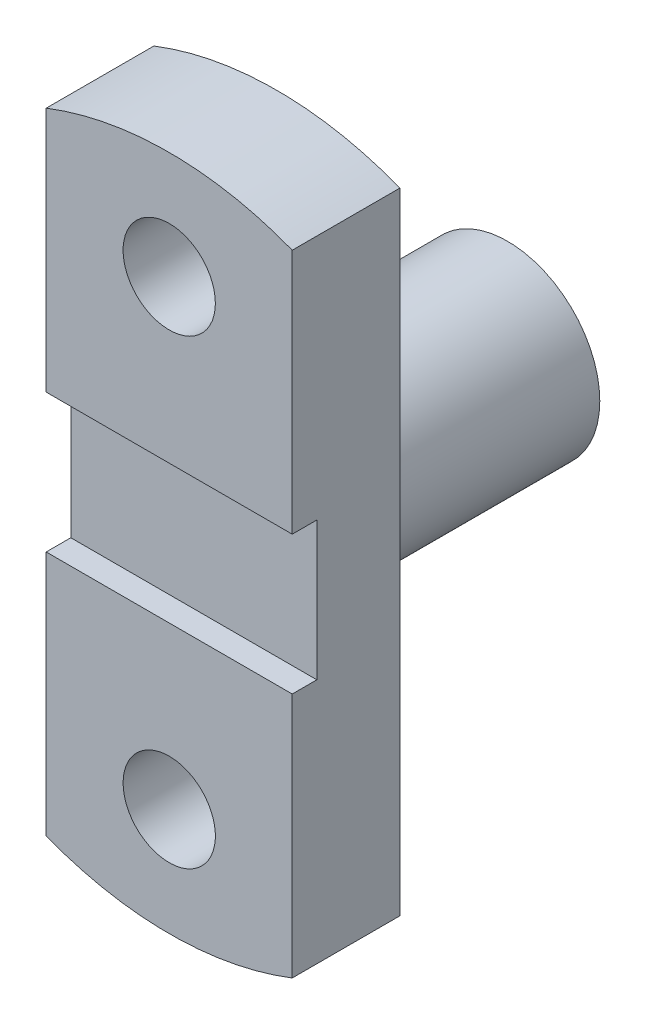
SolidWorks part; units mm, degrees
material "Alloy Steel"
ref_plane "Front Plane" through (0, 0, 0) normal (0, 0, 1) x (1, 0, 0)
ref_plane "Top Plane" through (0, 0, 0) normal (0, 1, 0) x (1, 0, 0)
ref_plane "Right Plane" through (0, 0, 0) normal (1, 0, 0) x (0, 0, -1)
sketch "Plate Profile Sketch" plane through (0, 0, 0) normal (0, 0, 1) x (1, 0, 0)
  line L0 (0, 0) -> (-208.7655, 0) construction
  line L2 (-40, -102.4695) -> (-40, 102.4695)
  line L4 (40, -102.4695) -> (40, 102.4695)
  line L5 (-40, -102.4695) -> (40, 102.4695) construction
  line L6 (-40, 102.4695) -> (40, -102.4695) construction
  arc A0 (-40, 102.4695) -> (40, 102.4695) centre (0, 0) cw
  arc A1 (-40, -102.4695) -> (40, -102.4695) centre (0, 0) ccw
  circle A2 centre (0, 75) radius 15
  circle A3 centre (0, -75) radius 15
  point P0 (0, 0)
  point P10 (0, 110)
  point P11 (0, -110)
  dimension "D1" = 110
  dimension "D4" = 30
  dimension "D2" = 80
  dimension "D3" = 220
  dimension "D5" = 75
extrude "Keeper Plate Body" add sketch "Plate Profile Sketch" along normal mid plane 35
sketch "Mounting Holes Sketch" plane through (40, 0, 0) normal (1, 0, 0) x (0, 0, -1)
  line L0 (-17.5, 22.5) -> (-9.5, 22.5)
  line L1 (-17.5, -102.4695) -> (-17.5, 102.4695) construction
  line L2 (-9.5, 22.5) -> (-9.5, -22.5)
  line L3 (-9.5, -22.5) -> (-17.5, -22.5)
  line L4 (-17.5, 22.5) -> (-17.5, -22.5)
  point P4 (-17.5, 0)
  dimension "D1" = 8
  dimension "D2" = 22.5
extrude "Mounting Holes" cut sketch "Mounting Holes Sketch" against normal up to surface (80 mm away) up to face at (-40, 0, 0)
sketch "Boss Ø60 Sketch" plane through (0, 0, -17.5) normal (0, 0, -1) x (-1, 0, 0)
  circle A0 centre (0, 0) radius 30
  dimension "D1" = 60
extrude "Cylindrical Boss Ø60" add sketch "Boss Ø60 Sketch" along normal blind 75
